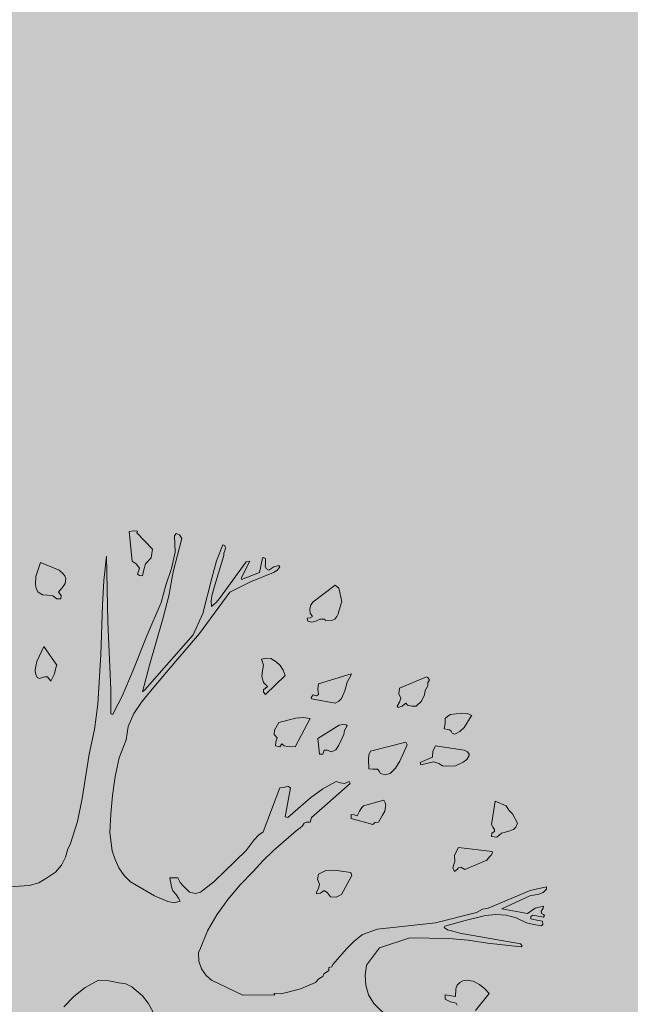
# Model space of a CAD drawing. Units: inches. Extents: x 84 to 1044, y -280 to 906.
# Tile 33 of 105: x 822 to 848, y -108 to -66. Entities that reach past the tile are written whole.
import ezdxf

# ---------------------------------------------------------------- set-up
doc = ezdxf.new("R2010")
doc.units = ezdxf.units.IN
doc.layers.add('L-PLNT', color=114, linetype='Continuous', lineweight=15)
doc.layers.add('L-PLNT-PATT', color=9, linetype='Continuous', lineweight=9, true_color=0xafd9aa)

# ---------------------------------------------------------------- blocks, each defined once
blk = doc.blocks.new('A$C37E508DF')
for p, q in [((0.6329, 1.5111), (0.6367, 1.5175)), ((0.6367, 1.5175), (0.6423, 1.5201)), ((0.6423, 1.5201), (0.6453, 1.5158)), ((0.6453, 1.5158), (0.644, 1.4879)), ((0.6826, 1.493), (0.7096, 1.5209)), ((0.7083, 1.5239), (0.7152, 1.5244)), ((0.7096, 1.5209), (0.7083, 1.5239)), ((0.7152, 1.5244), (0.7225, 1.5231)), ((0.7225, 1.5231), (0.7174, 1.4729)), ((0.5583, 1.4948), (0.5596, 1.4995)), ((0.5596, 1.4995), (0.563, 1.5003)), ((0.563, 1.5003), (0.5737, 1.4733)), ((0.6475, 1.4545), (0.6329, 1.5111)), ((0.4897, 1.4772), (0.4935, 1.4789)), ((0.4935, 1.4789), (0.4952, 1.478)), ((0.5596, 1.4905), (0.5583, 1.4948)), ((0.5613, 1.4862), (0.5596, 1.4905)), ((0.5608, 1.4823), (0.5613, 1.4862)), ((0.5767, 1.4317), (0.5608, 1.4823)), ((0.644, 1.4879), (0.6505, 1.46)), ((0.6852, 1.4785), (0.6826, 1.493)), ((0.7589, 1.3691), (0.7615, 1.481)), ((0.7615, 1.481), (0.7658, 1.4395)), ((0.4657, 1.4622), (0.4669, 1.4652)), ((0.4708, 1.4566), (0.4657, 1.4622)), ((0.4669, 1.4652), (0.4755, 1.463)), ((0.4755, 1.463), (0.4845, 1.4575)), ((0.4884, 1.4596), (0.4905, 1.4635)), ((0.4897, 1.4678), (0.4897, 1.4772)), ((0.4905, 1.4635), (0.4897, 1.4678)), ((0.4952, 1.478), (0.5004, 1.4532)), ((0.5313, 1.4437), (0.5167, 1.4729)), ((0.5167, 1.4729), (0.5231, 1.4716)), ((0.5231, 1.4716), (0.5686, 1.409)), ((0.5737, 1.4733), (0.5814, 1.4437)), ((0.6946, 1.4682), (0.6852, 1.4785)), ((0.6976, 1.4579), (0.6946, 1.4682)), ((0.7109, 1.4682), (0.7053, 1.4609)), ((0.7174, 1.4729), (0.7109, 1.4682)), ((0.8421, 1.4575), (0.8739, 1.4703)), ((0.8739, 1.4703), (0.882, 1.4463)), ((0.4764, 1.4532), (0.4708, 1.4566)), ((0.5154, 1.4373), (0.4764, 1.4532)), ((0.4845, 1.4575), (0.4884, 1.4596)), ((0.5004, 1.4532), (0.5308, 1.4412)), ((0.6552, 1.4137), (0.6475, 1.4545)), ((0.6505, 1.46), (0.6603, 1.4317)), ((0.7002, 1.4476), (0.6976, 1.4579)), ((0.7049, 1.448), (0.7002, 1.4476)), ((0.7083, 1.4502), (0.7049, 1.448)), ((0.7053, 1.4609), (0.7083, 1.4502)), ((0.831, 1.4424), (0.8323, 1.4476)), ((0.8323, 1.4476), (0.8357, 1.451)), ((0.8357, 1.451), (0.8421, 1.4575)), ((0.882, 1.4463), (0.8829, 1.433)), ((0.3649, 1.4266), (0.3709, 1.4317)), ((0.3709, 1.4317), (0.4086, 1.403)), ((0.551, 1.4197), (0.5154, 1.4373)), ((0.5308, 1.4412), (0.5313, 1.4437)), ((0.5814, 1.4133), (0.5767, 1.4317)), ((0.5814, 1.4437), (0.5969, 1.3833)), ((0.6603, 1.4317), (0.668, 1.4021)), ((0.7658, 1.4395), (0.7684, 1.3979)), ((0.8318, 1.4343), (0.831, 1.4424)), ((0.8353, 1.4292), (0.8318, 1.4343)), ((0.8434, 1.4197), (0.8353, 1.4292)), ((0.8829, 1.433), (0.8816, 1.4262)), ((0.3598, 1.403), (0.3628, 1.4189)), ((0.3628, 1.4189), (0.3649, 1.4266)), ((0.6029, 1.3494), (0.551, 1.4197)), ((0.5827, 1.4043), (0.5814, 1.4133)), ((0.6655, 1.3743), (0.6552, 1.4137)), ((0.8391, 1.4141), (0.8434, 1.4197)), ((0.8395, 1.4086), (0.8391, 1.4141)), ((0.8528, 1.4137), (0.846, 1.4086)), ((0.8619, 1.4146), (0.8528, 1.4137)), ((0.8709, 1.4154), (0.8619, 1.4146)), ((0.8781, 1.4197), (0.8709, 1.4154)), ((0.8816, 1.4262), (0.8781, 1.4197)), ((0.3602, 1.4021), (0.3598, 1.403)), ((0.364, 1.3888), (0.3602, 1.4021)), ((0.4086, 1.403), (0.4125, 1.3979)), ((0.4125, 1.3979), (0.4142, 1.391)), ((0.5686, 1.409), (0.5741, 1.4021)), ((0.5741, 1.4021), (0.5823, 1.3953)), ((0.5823, 1.3953), (0.5827, 1.4043)), ((0.668, 1.4021), (0.6925, 1.3455)), ((0.7684, 1.3979), (0.771, 1.3134)), ((0.846, 1.4086), (0.8395, 1.4086)), ((0.3657, 1.3828), (0.364, 1.3888)), ((0.3683, 1.3781), (0.3657, 1.3828)), ((0.3718, 1.3738), (0.3683, 1.3781)), ((0.4134, 1.3837), (0.4099, 1.3781)), ((0.4099, 1.3781), (0.4134, 1.376)), ((0.4142, 1.391), (0.4134, 1.3837)), ((0.5969, 1.3833), (0.6132, 1.3472)), ((0.3765, 1.3713), (0.3718, 1.3738)), ((0.3872, 1.3708), (0.3765, 1.3713)), ((0.3885, 1.3738), (0.3872, 1.3708)), ((0.3971, 1.3734), (0.3885, 1.3738)), ((0.4039, 1.3704), (0.3971, 1.3734)), ((0.4108, 1.3683), (0.4039, 1.3704)), ((0.4176, 1.37), (0.4108, 1.3683)), ((0.4134, 1.376), (0.4189, 1.3751)), ((0.4189, 1.3751), (0.4176, 1.37)), ((0.6882, 1.2949), (0.6655, 1.3743)), ((0.7538, 1.2529), (0.7589, 1.3691)), ((0.6595, 1.2829), (0.6029, 1.3494)), ((0.6132, 1.3472), (0.6959, 1.2529)), ((0.6925, 1.3455), (0.7161, 1.2868)), ((0.771, 1.3134), (0.7761, 1.2285)), ((0.846, 1.2949), (0.8687, 1.3271)), ((0.8687, 1.3271), (0.8803, 1.3014)), ((0.4597, 1.2868), (0.4648, 1.2945)), ((0.4648, 1.2945), (0.4717, 1.3009)), ((0.4717, 1.3009), (0.4807, 1.3065)), ((0.4807, 1.3065), (0.4884, 1.3074)), ((0.4884, 1.3074), (0.4965, 1.3057)), ((0.4965, 1.3057), (0.4935, 1.2954)), ((0.4935, 1.2954), (0.4948, 1.2855)), ((0.7002, 1.2495), (0.6882, 1.2949)), ((0.8473, 1.2924), (0.846, 1.2949)), ((0.8803, 1.3014), (0.8833, 1.2872)), ((0.3439, 1.2804), (0.3992, 1.2636)), ((0.3439, 1.2787), (0.3439, 1.2804)), ((0.3507, 1.2662), (0.3439, 1.2787)), ((0.4562, 1.2774), (0.4597, 1.2868)), ((0.4897, 1.2452), (0.4562, 1.2774)), ((0.4948, 1.2855), (0.4961, 1.2756)), ((0.6865, 1.2508), (0.6595, 1.2829)), ((0.7161, 1.2868), (0.7349, 1.2422)), ((0.8507, 1.2795), (0.8473, 1.2924)), ((0.8567, 1.2679), (0.8507, 1.2795)), ((0.8829, 1.2808), (0.8799, 1.2744)), ((0.8833, 1.2872), (0.8829, 1.2808)), ((0.2101, 1.2696), (0.2127, 1.2744)), ((0.2127, 1.2654), (0.2101, 1.2696)), ((0.2127, 1.2744), (0.2152, 1.2752)), ((0.2127, 1.2602), (0.2127, 1.2654)), ((0.2174, 1.2521), (0.2127, 1.2602)), ((0.2152, 1.2752), (0.2611, 1.2559)), ((0.3546, 1.2516), (0.3507, 1.2662)), ((0.3992, 1.2636), (0.4005, 1.2546)), ((0.4935, 1.2658), (0.4867, 1.2589)), ((0.4961, 1.2756), (0.4935, 1.2658)), ((0.8619, 1.2752), (0.8567, 1.2679)), ((0.867, 1.2752), (0.8619, 1.2752)), ((0.8713, 1.2739), (0.867, 1.2752)), ((0.8756, 1.2726), (0.8713, 1.2739)), ((0.8799, 1.2744), (0.8756, 1.2726)), ((0.2182, 1.2443), (0.2174, 1.2521)), ((0.2234, 1.2336), (0.2182, 1.2443)), ((0.262, 1.2465), (0.2586, 1.2388)), ((0.2611, 1.2559), (0.262, 1.2465)), ((0.3602, 1.2383), (0.3546, 1.2516)), ((0.4005, 1.2546), (0.3992, 1.2452)), ((0.3992, 1.2452), (0.4026, 1.2431)), ((0.4026, 1.2431), (0.4086, 1.2443)), ((0.4086, 1.2443), (0.4121, 1.2401)), ((0.4867, 1.2589), (0.4935, 1.2529)), ((0.4931, 1.2491), (0.4897, 1.2452)), ((0.4935, 1.2529), (0.4931, 1.2491)), ((0.7015, 1.2323), (0.6865, 1.2508)), ((0.6959, 1.2529), (0.7002, 1.2495)), ((0.7538, 1.2122), (0.7538, 1.2529)), ((0.2328, 1.2251), (0.2234, 1.2336)), ((0.2474, 1.2268), (0.2401, 1.2251)), ((0.2504, 1.2306), (0.2474, 1.2268)), ((0.2568, 1.2255), (0.2504, 1.2306)), ((0.2586, 1.2388), (0.2611, 1.2319)), ((0.2611, 1.2319), (0.265, 1.2251)), ((0.3649, 1.2336), (0.3602, 1.2383)), ((0.3709, 1.2306), (0.3649, 1.2336)), ((0.4112, 1.2375), (0.3709, 1.2306)), ((0.4121, 1.2401), (0.4112, 1.2375)), ((0.7148, 1.2126), (0.7015, 1.2323)), ((0.7349, 1.2422), (0.7482, 1.216)), ((0.7761, 1.2285), (0.7821, 1.1856)), ((0.1376, 1.2092), (0.1458, 1.2126)), ((0.1458, 1.2126), (0.1548, 1.2135)), ((0.1548, 1.2135), (0.1741, 1.2109)), ((0.1741, 1.2109), (0.1784, 1.2083)), ((0.2401, 1.2251), (0.2328, 1.2251)), ((0.2633, 1.2229), (0.2568, 1.2255)), ((0.265, 1.2251), (0.2633, 1.2229)), ((0.7246, 1.1908), (0.7148, 1.2126)), ((0.7482, 1.216), (0.7508, 1.2109)), ((0.7508, 1.2109), (0.7538, 1.2122)), ((0.1389, 1.2079), (0.1376, 1.2092)), ((0.1505, 1.189), (0.1389, 1.2079)), ((0.1784, 1.2083), (0.1831, 1.204)), ((0.1831, 1.204), (0.1831, 1.1959)), ((0.1831, 1.1959), (0.1848, 1.1865)), ((0.3507, 1.1916), (0.352, 1.1933)), ((0.352, 1.1933), (0.3576, 1.1942)), ((0.3576, 1.1942), (0.364, 1.1929)), ((0.364, 1.1929), (0.4005, 1.1702)), ((0.4134, 1.204), (0.4258, 1.2058)), ((0.4391, 1.156), (0.4134, 1.204)), ((0.4258, 1.2058), (0.4382, 1.2045)), ((0.4382, 1.2045), (0.4669, 1.1972)), ((0.4669, 1.1972), (0.4747, 1.1843)), ((0.1582, 1.1822), (0.1505, 1.189)), ((0.1668, 1.1775), (0.1582, 1.1822)), ((0.1711, 1.1792), (0.1668, 1.1775)), ((0.1728, 1.1826), (0.1711, 1.1792)), ((0.1758, 1.1847), (0.1728, 1.1826)), ((0.1788, 1.1852), (0.1758, 1.1847)), ((0.1848, 1.1865), (0.1788, 1.1852)), ((0.355, 1.1839), (0.3507, 1.1916)), ((0.3563, 1.177), (0.355, 1.1839)), ((0.3645, 1.1586), (0.3563, 1.177)), ((0.4751, 1.177), (0.47, 1.1714)), ((0.4747, 1.1843), (0.4751, 1.177)), ((0.7281, 1.168), (0.7246, 1.1908)), ((0.7821, 1.1856), (0.7911, 1.1436)), ((0.2478, 1.1594), (0.2504, 1.1637)), ((0.2607, 1.1316), (0.2478, 1.1594)), ((0.2504, 1.1637), (0.3104, 1.1487)), ((0.4005, 1.1702), (0.3979, 1.1436)), ((0.4622, 1.1607), (0.458, 1.1573)), ((0.4657, 1.156), (0.4622, 1.1607)), ((0.47, 1.1714), (0.4721, 1.1646)), ((0.4721, 1.1646), (0.473, 1.1573)), ((0.7396, 1.1371), (0.7281, 1.168)), ((0.1419, 1.1436), (0.1449, 1.1474)), ((0.1419, 1.141), (0.1419, 1.1436)), ((0.1449, 1.1474), (0.1509, 1.1504)), ((0.1509, 1.1504), (0.1994, 1.1573)), ((0.1994, 1.1573), (0.2041, 1.1479)), ((0.2041, 1.1479), (0.2045, 1.138)), ((0.3104, 1.1487), (0.3134, 1.1423)), ((0.37, 1.1509), (0.3645, 1.1586)), ((0.3778, 1.1474), (0.37, 1.1509)), ((0.3842, 1.15), (0.3778, 1.1474)), ((0.3898, 1.15), (0.3842, 1.15)), ((0.3923, 1.1436), (0.3898, 1.15)), ((0.3979, 1.1436), (0.3923, 1.1436)), ((0.4519, 1.1564), (0.4391, 1.156)), ((0.458, 1.1573), (0.4519, 1.1564)), ((0.473, 1.1573), (0.4657, 1.156)), ((0.7911, 1.1436), (0.8027, 1.0677)), ((0.1462, 1.1342), (0.1419, 1.141)), ((0.1522, 1.1294), (0.1462, 1.1342)), ((0.1655, 1.1234), (0.1522, 1.1294)), ((0.1938, 1.1273), (0.1878, 1.1234)), ((0.2032, 1.1303), (0.1938, 1.1273)), ((0.2247, 1.1251), (0.2032, 1.1303)), ((0.2045, 1.138), (0.226, 1.129)), ((0.226, 1.129), (0.2247, 1.1251)), ((0.268, 1.1196), (0.2607, 1.1316)), ((0.3134, 1.1423), (0.3139, 1.1346)), ((0.3139, 1.1346), (0.3134, 1.1183)), ((0.7469, 1.1054), (0.7396, 1.1371)), ((0.181, 1.1226), (0.1655, 1.1234)), ((0.1878, 1.1234), (0.181, 1.1226)), ((0.277, 1.1101), (0.268, 1.1196)), ((0.2856, 1.108), (0.277, 1.1101)), ((0.2933, 1.1101), (0.2856, 1.108)), ((0.2959, 1.1144), (0.2933, 1.1101)), ((0.2984, 1.1179), (0.2959, 1.1144)), ((0.3066, 1.1179), (0.2984, 1.1179)), ((0.3134, 1.1183), (0.3066, 1.1179)), ((0.3456, 1.093), (0.3469, 1.0964)), ((0.3842, 1.0591), (0.3456, 1.093)), ((0.3469, 1.0964), (0.355, 1.093)), ((0.355, 1.093), (0.3619, 1.0943)), ((0.3619, 1.0943), (0.3692, 1.0968)), ((0.3692, 1.0968), (0.3923, 1.0844)), ((0.7512, 1.0728), (0.7469, 1.1054)), ((0.3923, 1.0844), (0.4129, 1.069)), ((0.4472, 1.0857), (0.4515, 1.0887)), ((0.4562, 1.0364), (0.4472, 1.0857)), ((0.4515, 1.0887), (0.4584, 1.0865)), ((0.4584, 1.0865), (0.4657, 1.0861)), ((0.4657, 1.0861), (0.4939, 1.0107)), ((0.0789, 1.0552), (0.0978, 1.063)), ((0.0978, 1.063), (0.1042, 1.0231)), ((0.2847, 1.0565), (0.2856, 1.0604)), ((0.2856, 1.0604), (0.2877, 1.0647)), ((0.2877, 1.0647), (0.3224, 1.0552)), ((0.4112, 1.0351), (0.3842, 1.0591)), ((0.4129, 1.069), (0.4515, 1.0351)), ((0.7538, 1.0415), (0.7512, 1.0728)), ((0.8027, 1.0677), (0.8108, 1.0287)), ((0.0682, 1.0415), (0.0746, 1.0475)), ((0.0746, 1.0475), (0.0789, 1.0552)), ((0.2851, 1.054), (0.2847, 1.0565)), ((0.2864, 1.0463), (0.2851, 1.054)), ((0.2899, 1.039), (0.2864, 1.0463)), ((0.3224, 1.0552), (0.3255, 1.0522)), ((0.3255, 1.0522), (0.3293, 1.0458)), ((0.3293, 1.0458), (0.3336, 1.0381)), ((0.0596, 1.0257), (0.0682, 1.0415)), ((0.0626, 1.0188), (0.0596, 1.0257)), ((0.2972, 1.0274), (0.2899, 1.039)), ((0.3032, 1.0265), (0.2972, 1.0274)), ((0.3066, 1.0231), (0.3032, 1.0265)), ((0.3439, 1.0338), (0.3066, 1.0231)), ((0.3336, 1.0381), (0.3383, 1.0398)), ((0.3383, 1.0398), (0.3439, 1.0402)), ((0.3439, 1.0402), (0.3439, 1.0338)), ((0.4138, 1.0274), (0.4112, 1.0351)), ((0.4202, 1.0274), (0.4138, 1.0274)), ((0.4241, 1.0257), (0.4202, 1.0274)), ((0.4267, 1.0209), (0.4241, 1.0257)), ((0.4515, 1.0351), (0.4562, 1.0364)), ((0.7559, 1.0098), (0.7538, 1.0415)), ((0.8108, 1.0287), (0.8233, 0.9892)), ((0.0665, 1.0149), (0.0626, 1.0188)), ((0.0763, 1.0111), (0.0665, 1.0149)), ((0.087, 1.0085), (0.0763, 1.0111)), ((0.0948, 1.0016), (0.087, 1.0085)), ((0.1012, 1.018), (0.099, 1.0149)), ((0.099, 1.0149), (0.099, 1.0111)), ((0.099, 1.0111), (0.1033, 1.0085)), ((0.1042, 1.0231), (0.1012, 1.018)), ((0.1033, 1.0085), (0.1042, 1.0029)), ((0.4305, 1.0175), (0.4267, 1.0209)), ((0.4378, 1.0124), (0.4305, 1.0175)), ((0.476, 0.9789), (0.4378, 1.0124)), ((0.4939, 1.0107), (0.5021, 1.0051)), ((0.7516, 0.9785), (0.7559, 1.0098)), ((0.1042, 1.0029), (0.0948, 1.0016)), ((0.5021, 1.0051), (0.5094, 0.9969)), ((0.5094, 0.9969), (0.5231, 0.9789)), ((0.1025, 0.9751), (0.1029, 0.9772)), ((0.1046, 0.9708), (0.1025, 0.9751)), ((0.1029, 0.9772), (0.1604, 0.9841)), ((0.1604, 0.9841), (0.1672, 0.9708)), ((0.4939, 0.9618), (0.476, 0.9789)), ((0.5231, 0.9789), (0.578, 0.9253)), ((0.7469, 0.9635), (0.7516, 0.9785)), ((0.8233, 0.9892), (0.8275, 0.9815)), ((0.8275, 0.9815), (0.8314, 0.9673)), ((0.1076, 0.9682), (0.1046, 0.9708)), ((0.1119, 0.9626), (0.1076, 0.9682)), ((0.1496, 0.9463), (0.1119, 0.9626)), ((0.1672, 0.9708), (0.1664, 0.9601)), ((0.1664, 0.9601), (0.1698, 0.9493)), ((0.5111, 0.9429), (0.4939, 0.9618)), ((0.7401, 0.9493), (0.7469, 0.9635)), ((0.8314, 0.9673), (0.8383, 0.954)), ((0.1565, 0.9506), (0.1496, 0.9463)), ((0.1604, 0.9493), (0.1565, 0.9506)), ((0.1629, 0.9468), (0.1604, 0.9493)), ((0.1672, 0.9429), (0.1629, 0.9468)), ((0.1698, 0.9493), (0.1672, 0.9429)), ((0.3426, 0.936), (0.3443, 0.9412)), ((0.3443, 0.9412), (0.3722, 0.9451)), ((0.3722, 0.9451), (0.3868, 0.9446)), ((0.3868, 0.9446), (0.3992, 0.9386)), ((0.5334, 0.9202), (0.5111, 0.9429)), ((0.7315, 0.9365), (0.7401, 0.9493)), ((0.8383, 0.954), (0.8486, 0.942)), ((0.8486, 0.942), (0.8619, 0.933)), ((0.3602, 0.9039), (0.3426, 0.936)), ((0.4009, 0.9292), (0.3975, 0.9215)), ((0.3992, 0.9386), (0.4009, 0.9292)), ((0.578, 0.9253), (0.6011, 0.9077)), ((0.6303, 0.9189), (0.6359, 0.9245)), ((0.6359, 0.9245), (0.6397, 0.9322)), ((0.6397, 0.9322), (0.653, 0.9322)), ((0.653, 0.9322), (0.6505, 0.9172)), ((0.6796, 0.9013), (0.7203, 0.9253)), ((0.7203, 0.9253), (0.7315, 0.9365)), ((0.8619, 0.933), (0.8769, 0.9236)), ((0.0103, 0.9129), (0.0103, 0.9172)), ((0.0103, 0.9172), (0.0382, 0.9107)), ((0.0159, 0.9073), (0.0103, 0.9129)), ((0.0232, 0.9043), (0.0159, 0.9073)), ((0.0382, 0.9107), (0.1098, 0.8807)), ((0.3898, 0.9107), (0.3838, 0.9069)), ((0.3958, 0.906), (0.3898, 0.9107)), ((0.3975, 0.9215), (0.3996, 0.9142)), ((0.3996, 0.9142), (0.4031, 0.9077)), ((0.4031, 0.9077), (0.4026, 0.9052)), ((0.554, 0.8953), (0.5334, 0.9202)), ((0.6011, 0.9077), (0.6097, 0.9056)), ((0.6097, 0.9056), (0.6196, 0.9077)), ((0.6196, 0.9077), (0.6303, 0.9189)), ((0.6479, 0.9103), (0.6423, 0.9039)), ((0.6505, 0.9172), (0.6479, 0.9103)), ((0.8769, 0.9236), (0.8936, 0.9193)), ((0.8936, 0.9193), (0.9279, 0.9172)), ((0.0386, 0.9013), (0.0232, 0.9043)), ((0.0866, 0.8794), (0.0386, 0.9013)), ((0.3692, 0.8992), (0.3602, 0.9039)), ((0.379, 0.9), (0.3692, 0.8992)), ((0.3838, 0.9069), (0.379, 0.9)), ((0.4026, 0.9052), (0.3958, 0.906)), ((0.5728, 0.8691), (0.554, 0.8953)), ((0.6384, 0.8974), (0.6359, 0.8927)), ((0.6359, 0.8927), (0.6457, 0.8897)), ((0.6423, 0.9039), (0.6384, 0.8974)), ((0.6457, 0.8897), (0.6569, 0.8919)), ((0.6569, 0.8919), (0.6796, 0.9013)), ((0.0159, 0.8803), (0.0154, 0.8837)), ((0.0154, 0.8837), (0.0292, 0.8803)), ((0.0176, 0.8777), (0.0159, 0.8803)), ((0.0193, 0.8752), (0.0176, 0.8777)), ((0.0184, 0.8717), (0.0193, 0.8752)), ((0.0292, 0.8803), (0.0424, 0.8717)), ((0.0424, 0.8717), (0.0866, 0.8794)), ((0.1098, 0.8807), (0.1196, 0.8786)), ((0.1196, 0.8786), (0.1295, 0.873)), ((0.0133, 0.8679), (0.015, 0.87)), ((0.0154, 0.8649), (0.0133, 0.8679)), ((0.015, 0.87), (0.0184, 0.8717)), ((0.0334, 0.8687), (0.0154, 0.8649)), ((0.0163, 0.8529), (0.0171, 0.8584)), ((0.0171, 0.8584), (0.0266, 0.8602)), ((0.0266, 0.8602), (0.0369, 0.8623)), ((0.0369, 0.8666), (0.0334, 0.8687)), ((0.0369, 0.8623), (0.0369, 0.8666)), ((0.0617, 0.864), (0.0442, 0.8554)), ((0.0789, 0.8687), (0.0617, 0.864)), ((0.0965, 0.8696), (0.0789, 0.8687)), ((0.1141, 0.8679), (0.0965, 0.8696)), ((0.1492, 0.8593), (0.1141, 0.8679)), ((0.1295, 0.873), (0.1994, 0.8554)), ((0.1835, 0.8499), (0.1492, 0.8593)), ((0.5887, 0.8421), (0.5728, 0.8691)), ((0.0184, 0.8503), (0.0163, 0.8529)), ((0.0317, 0.8524), (0.0184, 0.8503)), ((0.0442, 0.8554), (0.0317, 0.8524)), ((0.1578, 0.8378), (0.1698, 0.8413)), ((0.1698, 0.8413), (0.1792, 0.8434)), ((0.1792, 0.8434), (0.1848, 0.8477)), ((0.1848, 0.8477), (0.1835, 0.8499)), ((0.1994, 0.8554), (0.2984, 0.8447)), ((0.2984, 0.8447), (0.3242, 0.8357)), ((0.6007, 0.8125), (0.5887, 0.8421)), ((0.0545, 0.8194), (0.1578, 0.8378)), ((0.1441, 0.8258), (0.1111, 0.8207)), ((0.1771, 0.8288), (0.1441, 0.8258)), ((0.2436, 0.8301), (0.1771, 0.8288)), ((0.2954, 0.813), (0.2436, 0.8301)), ((0.3242, 0.8357), (0.3387, 0.8241)), ((0.3387, 0.8241), (0.3512, 0.8117)), ((0.0519, 0.8164), (0.0545, 0.8194)), ((0.0532, 0.8143), (0.0519, 0.8164)), ((0.1111, 0.8207), (0.0532, 0.8143)), ((0.3173, 0.7834), (0.2954, 0.813)), ((0.3512, 0.8117), (0.3748, 0.7842)), ((0.6046, 0.8048), (0.6007, 0.8125)), ((0.599, 0.777), (0.6037, 0.7903)), ((0.6037, 0.7903), (0.6046, 0.8048)), ((0.3199, 0.7662), (0.3173, 0.7834)), ((0.3748, 0.7842), (0.3765, 0.7804)), ((0.3765, 0.7804), (0.3816, 0.7791)), ((0.3816, 0.7791), (0.382, 0.7744)), ((0.382, 0.7744), (0.3859, 0.7714)), ((0.5913, 0.7658), (0.599, 0.777)), ((0.1351, 0.7559), (0.1471, 0.7577)), ((0.1471, 0.7577), (0.1527, 0.7568)), ((0.1527, 0.7568), (0.1578, 0.7538)), ((0.3186, 0.7491), (0.3199, 0.7662)), ((0.3859, 0.7714), (0.3902, 0.7684)), ((0.3902, 0.7684), (0.3919, 0.7641)), ((0.3919, 0.7641), (0.3988, 0.7598)), ((0.3988, 0.7598), (0.4043, 0.7538)), ((0.5287, 0.7319), (0.5823, 0.7577)), ((0.5823, 0.7577), (0.5913, 0.7658)), ((0.7577, 0.7568), (0.7401, 0.7534)), ((0.7752, 0.7577), (0.7577, 0.7568)), ((0.798, 0.7452), (0.7752, 0.7577)), ((0.1081, 0.7349), (0.1153, 0.7427)), ((0.1153, 0.7427), (0.1244, 0.7504)), ((0.1244, 0.7504), (0.1351, 0.7559)), ((0.1578, 0.7538), (0.1629, 0.7491)), ((0.1629, 0.7491), (0.1651, 0.7431)), ((0.1651, 0.7431), (0.1655, 0.7298)), ((0.3139, 0.7324), (0.3186, 0.7491)), ((0.4043, 0.7538), (0.4301, 0.7431)), ((0.4301, 0.7431), (0.4515, 0.7371)), ((0.7182, 0.7461), (0.7002, 0.7307)), ((0.7285, 0.7512), (0.7182, 0.7461)), ((0.7401, 0.7534), (0.7285, 0.7512)), ((0.8173, 0.7298), (0.798, 0.7452)), ((0.1312, 0.7058), (0.1081, 0.7349)), ((0.1655, 0.7298), (0.1831, 0.7324)), ((0.1831, 0.7255), (0.1741, 0.7208)), ((0.1831, 0.7324), (0.1831, 0.7255)), ((0.3049, 0.7178), (0.3139, 0.7324)), ((0.4515, 0.7371), (0.4635, 0.7341)), ((0.4635, 0.7341), (0.4755, 0.7349)), ((0.4755, 0.7349), (0.4742, 0.7324)), ((0.4742, 0.7324), (0.5287, 0.7319)), ((0.7002, 0.7307), (0.6903, 0.7186)), ((0.8344, 0.7122), (0.8173, 0.7298)), ((0.1646, 0.7186), (0.1629, 0.7152)), ((0.1741, 0.7208), (0.1646, 0.7186)), ((0.28, 0.6933), (0.3049, 0.7178)), ((0.6903, 0.7186), (0.6818, 0.7032))]:
    blk.add_line(p, q)

msp = doc.modelspace()

# ---------------------------------------------------------------- hatches: boundary and pattern name
at = {"layer": 'L-PLNT-PATT', "transparency": 33554597}
h = msp.add_hatch(color=256, dxfattribs=at)
h.dxf.hatch_style = 1
h.paths.add_polyline_path([(791.074, 31.12), (791.074, 91.12), (743.074, 91.12), (674.074, 91.12), (674.074, 31.12), (650.074, 31.12), (650.074, -112.88), (983.074, -112.88), (983.074, -64.88), (791.074, -64.88)])

# ---------------------------------------------------------------- block references
at = {"layer": 'L-PLNT', "xscale": -24.64361536662419, "yscale": 24.64361536662419, "zscale": 24.64361536662419}
msp.add_blockref('A$C37E508DF', (844.575, -125.52), dxfattribs=at)

doc.saveas('drawing.dxf')
